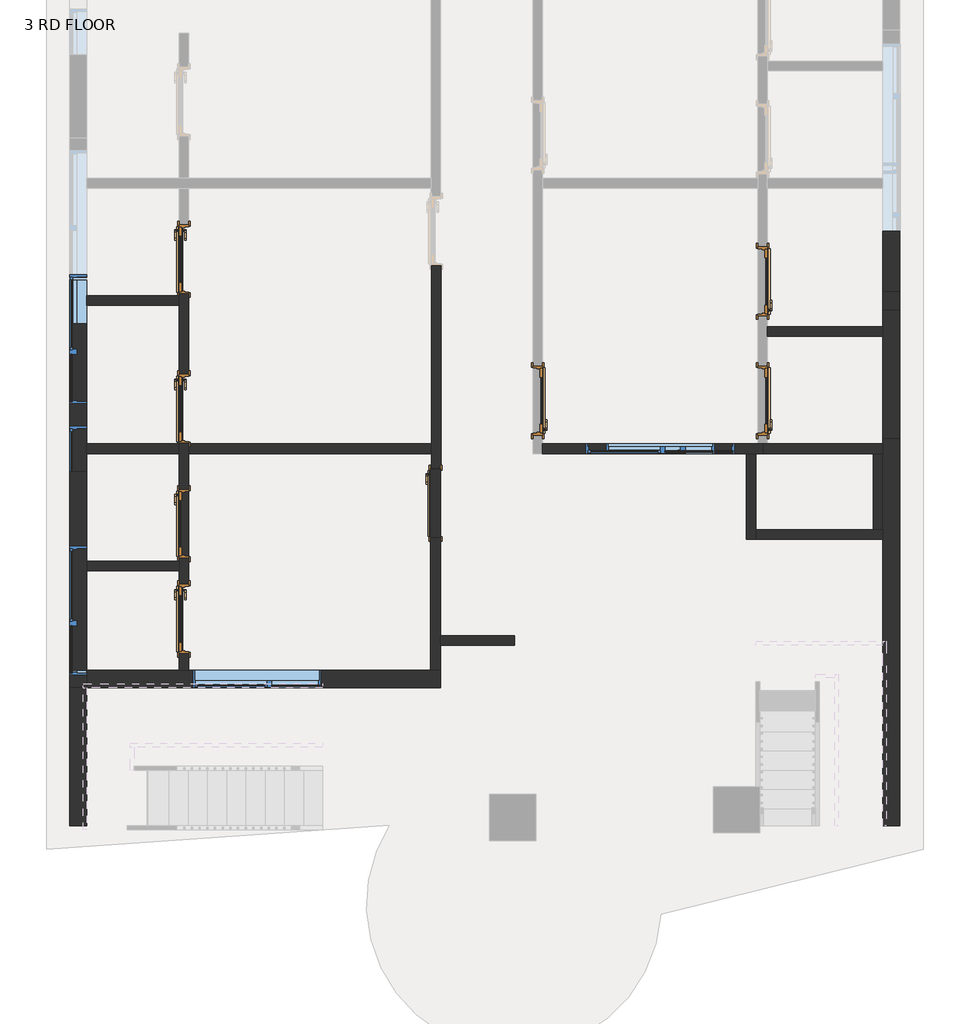
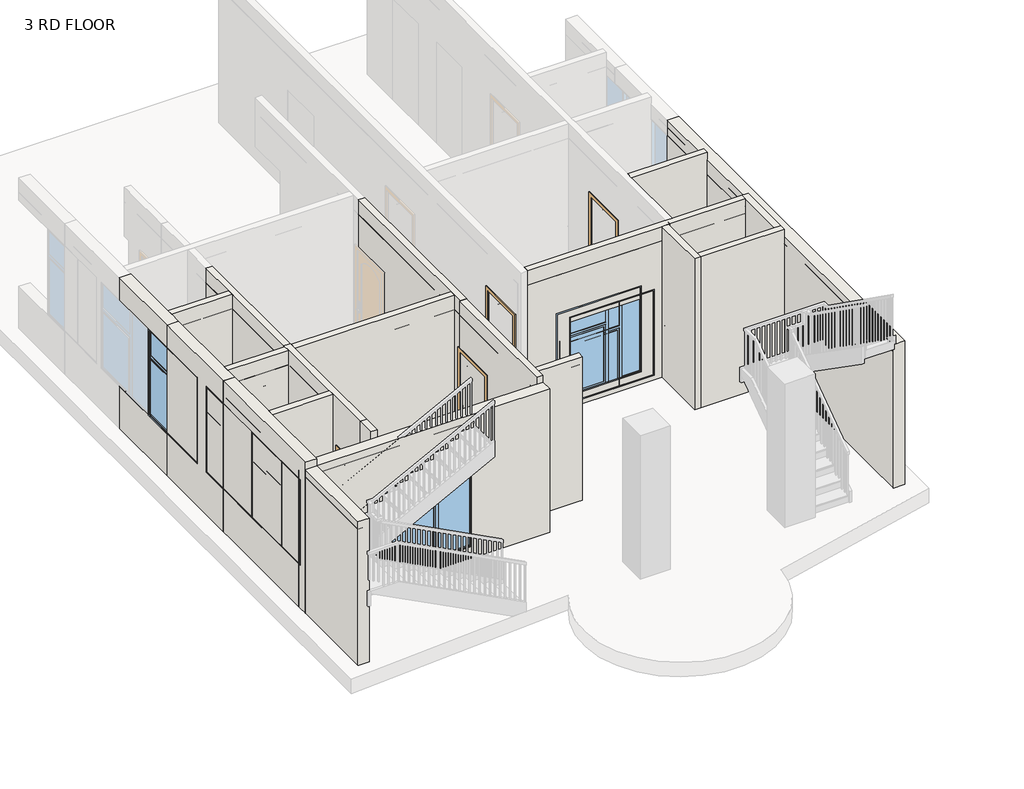
# One storey, part 1 of 5: 41 walls, 8 doors, 7 windows.
"""IFC4 building model written with IfcOpenShell, lengths in millimetres."""

from ifc_helpers import new_model, si_unit, frame, origin, place, context, project, spatial, polyline, outline, extrude, faceted_brep, transform, mapped, element, save
from components import door_346b4a94, m_window_casement_double_sidelight_1702_x_1829mm_c8b42c7f, m_window_casement_double_sidelight_1702_x_1829mm_92594323

model = new_model("IFC4")

# Units and contexts
model_context = context("Model", 3, world=origin())
ifc_project = project(units=[si_unit("LENGTHUNIT", "METRE", prefix="MILLI")], contexts=[model_context])

# Site, building, storey
site = spatial("IfcSite", under=ifc_project)
building = spatial("IfcBuilding", under=site)
storey = spatial("IfcBuildingStorey", under=building, Name="3 RD FLOOR", Elevation=9601.2)

# Doors
placement = place(None, origin())
door_shape = door_346b4a94(model_context)
element("IfcDoor", 1, ObjectType="2'10\"X7'", at=placement, inside=storey, context=model_context, shape_type="MappedRepresentation", body=[
    mapped(door_shape, transform((2698.7641134, -459.3600272, 9601.2), x_axis=(0.0, -1.0, 0.0), y_axis=(1.0, 0.0, 0.0), z_axis=(0.0, 0.0, 1.0))),
])
element("IfcDoor", 2, ObjectType="2'10\"X7'", at=placement, inside=storey, context=model_context, shape_type="MappedRepresentation", body=[
    mapped(door_shape, transform((2698.7641134, -2034.1600272, 9601.2), x_axis=(0.0, -1.0, 0.0), y_axis=(1.0, 0.0, 0.0), z_axis=(0.0, 0.0, 1.0))),
])
element("IfcDoor", 3, ObjectType="2'10\"X7'", at=placement, inside=storey, context=model_context, shape_type="MappedRepresentation", body=[
    mapped(door_shape, transform((-273.0358866, -2034.1600272, 9601.2), x_axis=(0.0, -1.0, 0.0), y_axis=(1.0, 0.0, 0.0), z_axis=(0.0, 0.0, 1.0))),
])
element("IfcDoor", 4, ObjectType="2'10\"X7'", at=placement, inside=storey, context=model_context, shape_type="MappedRepresentation", body=[
    mapped(door_shape, transform((-4952.9858866, -3659.7600272, 9601.2), x_axis=(0.0, 1.0, 0.0), y_axis=(-1.0, 0.0, 0.0), z_axis=(0.0, 0.0, 1.0))),
])
element("IfcDoor", 5, ObjectType="2'10\"X7'", at=placement, inside=storey, context=model_context, shape_type="MappedRepresentation", body=[
    mapped(door_shape, transform((-4952.9858866, -2142.5151651, 9601.2), x_axis=(0.0, 1.0, 0.0), y_axis=(-1.0, 0.0, 0.0), z_axis=(0.0, 0.0, 1.0))),
])
element("IfcDoor", 6, ObjectType="2'10\"X7'", at=placement, inside=storey, context=model_context, shape_type="MappedRepresentation", body=[
    mapped(door_shape, transform((-4952.9858866, -167.9704957, 9601.2), x_axis=(0.0, 1.0, 0.0), y_axis=(-1.0, 0.0, 0.0), z_axis=(0.0, 0.0, 1.0))),
])
element("IfcDoor", 7, ObjectType="2'10\"X7'", at=placement, inside=storey, context=model_context, shape_type="MappedRepresentation", body=[
    mapped(door_shape, transform((-1629.1419858, -3390.4626067, 9601.2), x_axis=(0.0, 1.0, 0.0), y_axis=(-1.0, 0.0, 0.0), z_axis=(0.0, 0.0, 1.0))),
])
element("IfcDoor", 8, ObjectType="2'10\"X7'", at=placement, inside=storey, context=model_context, shape_type="MappedRepresentation", body=[
    mapped(door_shape, transform((-4952.9858866, -4917.0600272, 9601.2), x_axis=(0.0, 1.0, 0.0), y_axis=(-1.0, 0.0, 0.0), z_axis=(0.0, 0.0, 1.0))),
])

# Walls
element("IfcWall", 9, ObjectType="Generic - 4.5\"", at=placement, inside=storey, context=model_context, shape_type="SweptSolid", body=[
    extrude(outline(polyline([(-5013.3108866, -776.8600272), (-6232.5508078, -776.8600272), (-6232.5508078, -649.8600272), (-5013.3108866, -649.8600272), (-5013.3108866, -776.8600272)])), frame((0.0, 0.0, 9601.2), z_axis=(0.0, 0.0, 1.0), x_axis=(1.0, 0.0, 0.0)), (0.0, 0.0, 1.0), 3200.4),
])
element("IfcWall", 10, ObjectType="Generic - 4.5\"", at=placement, inside=storey, context=model_context, shape_type="Brep", body=[
    faceted_brep([(-5013.3108866, -2574.3151651, 12801.6), (-5013.3108866, -776.8600272, 12801.6), (-5013.3108866, -649.8600272, 12801.6), (-5013.3108866, 136.8295043, 12801.6), (-5013.3108866, 136.8295043, 12496.8), (-5013.3108866, 136.8295043, 11759.8), (-5013.3108866, -624.7704957, 11759.8), (-5013.3108866, -624.7704957, 9601.2), (-5013.3108866, -649.8600272, 9601.2), (-5013.3108866, -776.8600272, 9601.2), (-5013.3108866, -1685.7151651, 9601.2), (-5013.3108866, -1685.7151651, 11759.8), (-5013.3108866, -2574.3151651, 11759.8), (-5013.3108866, -2574.3151651, 12496.8), (-4886.3108866, 136.8295043, 12801.6), (-4886.3108866, -2574.3151651, 12801.6), (-4886.3108866, -2574.3151651, 12496.8), (-4886.3108866, -2574.3151651, 11759.8), (-4886.3108866, -1685.7151651, 11759.8), (-4886.3108866, -1685.7151651, 9601.2), (-4886.3108866, -624.7704957, 9601.2), (-4886.3108866, -624.7704957, 11759.8), (-4886.3108866, 136.8295043, 11759.8), (-4886.3108866, 136.8295043, 12496.8)], [[[0, 1, 2, 3, 4, 5, 6, 7, 8, 9, 10, 11, 12, 13]], [[14, 15, 16, 17, 18, 19, 20, 21, 22, 23]], [[19, 10, 9, 8, 7, 20]], [[3, 2, 1, 0, 15, 14]], [[18, 11, 10, 19]], [[11, 18, 17, 12]], [[21, 6, 5, 22]], [[6, 21, 20, 7]], [[15, 0, 13, 12, 17, 16]], [[3, 14, 23, 22, 5, 4]]]),
])
element("IfcWall", 11, ObjectType="Generic - 4.5\"", at=placement, inside=storey, context=model_context, shape_type="SweptSolid", body=[
    extrude(outline(polyline([(-5013.3108866, -2732.6600272), (-6232.5508078, -2732.6600272), (-6232.5508078, -2605.6600272), (-5013.3108866, -2605.6600272), (-5013.3108866, -2732.6600272)])), frame((0.0, 0.0, 9601.2), z_axis=(0.0, 0.0, 1.0), x_axis=(1.0, 0.0, 0.0)), (0.0, 0.0, 1.0), 3200.4),
])
element("IfcWall", 12, ObjectType="Generic - 4.5\"", at=placement, inside=storey, context=model_context, shape_type="Brep", body=[
    faceted_brep([(-5013.3108866, -5221.8600272, 12801.6), (-5013.3108866, -4282.0600272, 12801.6), (-5013.3108866, -4155.0600272, 12801.6), (-5013.3108866, -2732.6600272, 12801.6), (-5013.3108866, -2605.6600272, 12801.6), (-5013.3108866, -2574.3151651, 12801.6), (-5013.3108866, -2574.3151651, 12496.8), (-5013.3108866, -2574.3151651, 11759.8), (-5013.3108866, -2599.3151651, 11759.8), (-5013.3108866, -2599.3151651, 9601.2), (-5013.3108866, -2605.6600272, 9601.2), (-5013.3108866, -2732.6600272, 9601.2), (-5013.3108866, -3202.9600272, 9601.2), (-5013.3108866, -3202.9600272, 11759.8), (-5013.3108866, -4116.5600272, 11759.8), (-5013.3108866, -4116.5600272, 9601.2), (-5013.3108866, -4155.0600272, 9601.2), (-5013.3108866, -4282.0600272, 9601.2), (-5013.3108866, -4460.2600272, 9601.2), (-5013.3108866, -4460.2600272, 11759.8), (-5013.3108866, -5221.8600272, 11759.8), (-5013.3108866, -5221.8600272, 12496.8), (-4886.3108866, -2574.3151651, 12801.6), (-4886.3108866, -2605.6600272, 12801.6), (-4886.3108866, -2732.6600272, 12801.6), (-4886.3108866, -5221.8600272, 12801.6), (-4886.3108866, -5221.8600272, 12496.8), (-4886.3108866, -5221.8600272, 11759.8), (-4886.3108866, -4460.2600272, 11759.8), (-4886.3108866, -4460.2600272, 9601.2), (-4886.3108866, -4116.5600272, 9601.2), (-4886.3108866, -4116.5600272, 11759.8), (-4886.3108866, -3202.9600272, 11759.8), (-4886.3108866, -3202.9600272, 9601.2), (-4886.3108866, -2732.6600272, 9601.2), (-4886.3108866, -2605.6600272, 9601.2), (-4886.3108866, -2599.3151651, 9601.2), (-4886.3108866, -2599.3151651, 11759.8), (-4886.3108866, -2574.3151651, 11759.8), (-4886.3108866, -2574.3151651, 12496.8)], [[[0, 1, 2, 3, 4, 5, 6, 7, 8, 9, 10, 11, 12, 13, 14, 15, 16, 17, 18, 19, 20, 21]], [[22, 23, 24, 25, 26, 27, 28, 29, 30, 31, 32, 33, 34, 35, 36, 37, 38, 39]], [[33, 12, 11, 10, 9, 36, 35, 34]], [[15, 30, 29, 18, 17, 16]], [[5, 4, 3, 2, 1, 0, 25, 24, 23, 22]], [[32, 13, 12, 33]], [[13, 32, 31, 14]], [[14, 31, 30, 15]], [[37, 8, 7, 38]], [[8, 37, 36, 9]], [[28, 19, 18, 29]], [[19, 28, 27, 20]], [[5, 22, 39, 38, 7, 6]], [[25, 0, 21, 20, 27, 26]]]),
])
element("IfcWall", 13, ObjectType="Generic - 4.5\"", at=placement, inside=storey, context=model_context, shape_type="SweptSolid", body=[
    extrude(outline(polyline([(-5013.3108866, -4282.0600272), (-6232.5324766, -4282.0600272), (-6232.5342541, -4155.0600272), (-5013.3108866, -4155.0600272), (-5013.3108866, -4282.0600272)])), frame((0.0, 0.0, 9601.2), z_axis=(0.0, 0.0, 1.0), x_axis=(1.0, 0.0, 0.0)), (0.0, 0.0, 1.0), 3200.4),
])
element("IfcWall", 14, ObjectType="Generic - 4.5\"", at=placement, inside=storey, context=model_context, shape_type="SweptSolid", body=[
    extrude(outline(polyline([(-1685.9108866, -2732.6600272), (-4886.3108866, -2732.6600272), (-4886.3108866, -2605.6600272), (-1685.9108866, -2605.6600272), (-1685.9108866, -2732.6600272)])), frame((0.0, 0.0, 9601.2), z_axis=(0.0, 0.0, 1.0), x_axis=(1.0, 0.0, 0.0)), (0.0, 0.0, 1.0), 3200.4),
])
element("IfcWall", 15, ObjectType="Generic - 4.5\"", at=placement, inside=storey, context=model_context, shape_type="Brep", body=[
    faceted_brep([(-1680.4827262, -2933.2626067, 12801.6), (-1680.4827262, 609.3637706, 12801.6), (-1680.4827262, 609.3637706, 11759.8), (-1680.4827262, -253.8362294, 11759.8), (-1680.4827262, -253.8362294, 9601.2), (-1680.4827262, -2933.2626067, 9601.2), (-1553.4827262, 609.3637706, 12801.6), (-1553.4827262, -2933.2626067, 12801.6), (-1553.4827262, -2933.2626067, 9601.2), (-1553.4827262, -253.8362294, 9601.2), (-1553.4827262, -253.8362294, 11759.8), (-1553.4827262, 609.3637706, 11759.8), (-1562.4669858, -2933.2626067, 9601.2), (-1562.4669858, -2933.2626067, 12801.6), (-1558.4871817, 609.3637706, 12801.6), (-1558.4871817, 609.3637706, 11759.8)], [[[0, 1, 2, 3, 4, 5]], [[6, 7, 8, 9, 10, 11]], [[8, 12, 5, 4, 9]], [[1, 0, 13, 7, 6, 14]], [[10, 3, 2, 15, 11]], [[3, 10, 9, 4]], [[5, 12, 8, 7, 13, 0]], [[1, 14, 6, 11, 15, 2]]]),
])
element("IfcWall", 16, ObjectType="Generic - 4.5\"", at=placement, inside=storey, context=model_context, shape_type="Brep", body=[
    faceted_brep([(-1689.4669858, -5596.1082131, 12801.6), (-1689.4669858, -2933.2626067, 12801.6), (-1689.4669858, -2933.2626067, 9601.2), (-1689.4669858, -2933.6626067, 9601.2), (-1689.4669858, -2933.6626067, 11759.8), (-1689.4669858, -3847.2626067, 11759.8), (-1689.4669858, -3847.2626067, 9601.2), (-1689.4669858, -5596.1082131, 9601.2), (-1562.4669858, -2933.2626067, 12801.6), (-1562.4669858, -5596.1082131, 12801.6), (-1562.4669858, -5596.1082131, 12649.2), (-1562.4669858, -5596.1082131, 12496.8), (-1562.4669858, -5596.1082131, 9601.2), (-1562.4669858, -5263.3822004, 9601.2), (-1562.4669858, -5136.3822004, 9601.2), (-1562.4669858, -3847.2626067, 9601.2), (-1562.4669858, -3847.2626067, 11759.8), (-1562.4669858, -2933.6626067, 11759.8), (-1562.4669858, -2933.6626067, 9601.2), (-1562.4669858, -2933.2626067, 9601.2), (-1680.4827262, -2933.2626067, 9601.2), (-1680.4827262, -2933.2626067, 12801.6)], [[[0, 1, 2, 3, 4, 5, 6, 7]], [[8, 9, 10, 11, 12, 13, 14, 15, 16, 17, 18, 19]], [[2, 20, 19, 18, 3]], [[12, 7, 6, 15, 14, 13]], [[1, 0, 9, 8, 21]], [[17, 4, 3, 18]], [[4, 17, 16, 5]], [[5, 16, 15, 6]], [[7, 12, 11, 10, 9, 0]], [[1, 21, 8, 19, 20, 2]]]),
])
element("IfcWall", 17, ObjectType="Generic - 4.5\"", at=placement, inside=storey, context=model_context, shape_type="Brep", body=[
    faceted_brep([(-212.7108866, -2732.6600272, 12801.6), (-212.7108866, -2732.6600272, 9601.2), (2479.6891134, -2732.6600272, 9601.2), (2606.6891134, -2732.6600272, 9601.2), (4281.7311655, -2732.6600272, 9601.2), (4281.7311655, -2732.6600272, 12649.2), (4154.7311655, -2732.6600272, 12649.2), (4154.7311655, -2732.6600272, 12801.6), (2606.6891134, -2732.6600272, 12801.6), (2479.6891134, -2732.6600272, 12801.6), (358.7891134, -2732.6600272, 11691.1092519), (2060.5891134, -2732.6600272, 11691.1092519), (2060.5891134, -2732.6600272, 9862.3092519), (358.7891134, -2732.6600272, 9862.3092519), (-212.7108866, -2605.6600272, 9601.2), (-212.7108866, -2605.6600272, 12801.6), (2632.0891134, -2605.6600272, 12801.6), (2759.0891134, -2605.6600272, 12801.6), (4154.7311655, -2605.6600272, 12801.6), (4154.7311655, -2605.6600272, 12649.2), (4281.7311655, -2605.6600272, 12649.2), (4281.7311655, -2605.6600272, 9601.2), (2759.0891134, -2605.6600272, 9601.2), (2632.0891134, -2605.6600272, 9601.2), (358.7891134, -2605.6600272, 11691.1092519), (358.7891134, -2605.6600272, 9862.3092519), (2060.5891134, -2605.6600272, 9862.3092519), (2060.5891134, -2605.6600272, 11691.1092519)], [[[0, 1, 2, 3, 4, 5, 6, 7, 8, 9], [10, 11, 12, 13]], [[14, 15, 16, 17, 18, 19, 20, 21, 22, 23], [24, 25, 26, 27]], [[4, 3, 2, 1, 14, 23, 22, 21]], [[0, 9, 8, 7, 18, 17, 16, 15]], [[25, 24, 10, 13]], [[26, 25, 13, 12]], [[27, 26, 12, 11]], [[24, 27, 11, 10]], [[0, 15, 14, 1]], [[19, 6, 5, 20]], [[4, 21, 20, 5]], [[7, 6, 19, 18]]]),
])
element("IfcWall", 18, ObjectType="Generic - 4.5\"", at=placement, inside=storey, context=model_context, shape_type="SweptSolid", body=[
    extrude(outline(polyline([(4281.7311655, -1183.2600272), (2759.0891134, -1183.2600272), (2759.0891134, -1056.2600272), (4281.7311655, -1056.2600272), (4281.7311655, -1183.2600272)])), frame((0.0, 0.0, 9601.2), z_axis=(0.0, 0.0, 1.0), x_axis=(1.0, 0.0, 0.0)), (0.0, 0.0, 1.0), 3200.4),
])
element("IfcWall", 19, ObjectType="Generic - 4.5\"", at=placement, inside=storey, context=model_context, shape_type="SweptSolid", body=[
    extrude(outline(polyline([(-5013.3108866, -776.8600272), (-6232.5508078, -776.8600272), (-6232.5508078, -649.8600272), (-5013.3108866, -649.8600272), (-5013.3108866, -776.8600272)])), frame((0.0, 0.0, 9601.2), z_axis=(0.0, 0.0, 1.0), x_axis=(1.0, 0.0, 0.0)), (0.0, 0.0, 1.0), 2895.6),
])
element("IfcWall", 20, ObjectType="Generic - 4.5\"", at=placement, inside=storey, context=model_context, shape_type="Brep", body=[
    faceted_brep([(-5013.3108866, -2574.3151651, 12496.8), (-5013.3108866, -776.8600272, 12496.8), (-5013.3108866, -649.8600272, 12496.8), (-5013.3108866, 136.8295043, 12496.8), (-5013.3108866, 136.8295043, 11759.8), (-5013.3108866, -624.7704957, 11759.8), (-5013.3108866, -624.7704957, 9601.2), (-5013.3108866, -649.8600272, 9601.2), (-5013.3108866, -776.8600272, 9601.2), (-5013.3108866, -1685.7151651, 9601.2), (-5013.3108866, -1685.7151651, 11759.8), (-5013.3108866, -2574.3151651, 11759.8), (-4886.3108866, 136.8295043, 12496.8), (-4886.3108866, -2574.3151651, 12496.8), (-4886.3108866, -2574.3151651, 11759.8), (-4886.3108866, -1685.7151651, 11759.8), (-4886.3108866, -1685.7151651, 9601.2), (-4886.3108866, -624.7704957, 9601.2), (-4886.3108866, -624.7704957, 11759.8), (-4886.3108866, 136.8295043, 11759.8)], [[[0, 1, 2, 3, 4, 5, 6, 7, 8, 9, 10, 11]], [[12, 13, 14, 15, 16, 17, 18, 19]], [[16, 9, 8, 7, 6, 17]], [[13, 0, 11, 14]], [[3, 12, 19, 4]], [[3, 2, 1, 0, 13, 12]], [[18, 5, 4, 19]], [[5, 18, 17, 6]], [[15, 10, 9, 16]], [[10, 15, 14, 11]]]),
])
element("IfcWall", 21, ObjectType="Generic - 4.5\"", at=placement, inside=storey, context=model_context, shape_type="SweptSolid", body=[
    extrude(outline(polyline([(-5013.3108866, -2732.6600272), (-6232.5508078, -2732.6600272), (-6232.5508078, -2605.6600272), (-5013.3108866, -2605.6600272), (-5013.3108866, -2732.6600272)])), frame((0.0, 0.0, 9601.2), z_axis=(0.0, 0.0, 1.0), x_axis=(1.0, 0.0, 0.0)), (0.0, 0.0, 1.0), 2895.6),
])
element("IfcWall", 22, ObjectType="Generic - 4.5\"", at=placement, inside=storey, context=model_context, shape_type="Brep", body=[
    faceted_brep([(-5013.3108866, -5221.8600272, 12496.8), (-5013.3108866, -4282.0600272, 12496.8), (-5013.3108866, -4155.0600272, 12496.8), (-5013.3108866, -2732.6600272, 12496.8), (-5013.3108866, -2605.6600272, 12496.8), (-5013.3108866, -2574.3151651, 12496.8), (-5013.3108866, -2574.3151651, 11759.8), (-5013.3108866, -2599.3151651, 11759.8), (-5013.3108866, -2599.3151651, 9601.2), (-5013.3108866, -2605.6600272, 9601.2), (-5013.3108866, -2732.6600272, 9601.2), (-5013.3108866, -4155.0600272, 9601.2), (-5013.3108866, -4282.0600272, 9601.2), (-5013.3108866, -4460.2600272, 9601.2), (-5013.3108866, -4460.2600272, 11759.8), (-5013.3108866, -5221.8600272, 11759.8), (-4886.3108866, -2574.3151651, 12496.8), (-4886.3108866, -2605.6600272, 12496.8), (-4886.3108866, -2732.6600272, 12496.8), (-4886.3108866, -5221.8600272, 12496.8), (-4886.3108866, -5221.8600272, 11759.8), (-4886.3108866, -4460.2600272, 11759.8), (-4886.3108866, -4460.2600272, 9601.2), (-4886.3108866, -2732.6600272, 9601.2), (-4886.3108866, -2605.6600272, 9601.2), (-4886.3108866, -2599.3151651, 9601.2), (-4886.3108866, -2599.3151651, 11759.8), (-4886.3108866, -2574.3151651, 11759.8)], [[[0, 1, 2, 3, 4, 5, 6, 7, 8, 9, 10, 11, 12, 13, 14, 15]], [[16, 17, 18, 19, 20, 21, 22, 23, 24, 25, 26, 27]], [[8, 25, 24, 23, 22, 13, 12, 11, 10, 9]], [[19, 0, 15, 20]], [[5, 16, 27, 6]], [[5, 4, 3, 2, 1, 0, 19, 18, 17, 16]], [[21, 14, 13, 22]], [[14, 21, 20, 15]], [[26, 7, 6, 27]], [[7, 26, 25, 8]]]),
])
element("IfcWall", 23, ObjectType="Generic - 4.5\"", at=placement, inside=storey, context=model_context, shape_type="SweptSolid", body=[
    extrude(outline(polyline([(-5013.3108866, -4282.0600272), (-6232.5324766, -4282.0600272), (-6232.5342541, -4155.0600272), (-5013.3108866, -4155.0600272), (-5013.3108866, -4282.0600272)])), frame((0.0, 0.0, 9601.2), z_axis=(0.0, 0.0, 1.0), x_axis=(1.0, 0.0, 0.0)), (0.0, 0.0, 1.0), 2895.6),
])
element("IfcWall", 24, ObjectType="Generic - 4.5\"", at=placement, inside=storey, context=model_context, shape_type="SweptSolid", body=[
    extrude(outline(polyline([(-1685.9108866, -2732.6600272), (-4886.3108866, -2732.6600272), (-4886.3108866, -2605.6600272), (-1685.9108866, -2605.6600272), (-1685.9108866, -2732.6600272)])), frame((0.0, 0.0, 9601.2), z_axis=(0.0, 0.0, 1.0), x_axis=(1.0, 0.0, 0.0)), (0.0, 0.0, 1.0), 2895.6),
])
element("IfcWall", 25, ObjectType="Generic - 4.5\"", at=placement, inside=storey, context=model_context, shape_type="Brep", body=[
    faceted_brep([(-1680.4827262, -2933.2626067, 9601.2), (-1680.4827262, -2933.2626067, 12496.8), (-1680.4827262, 609.3637706, 12496.8), (-1680.4827262, 609.3637706, 11759.8), (-1680.4827262, -253.8362294, 11759.8), (-1680.4827262, -253.8362294, 9601.2), (-1553.4827262, -2933.2626067, 12496.8), (-1553.4827262, -2933.2626067, 9601.2), (-1553.4827262, -253.8362294, 9601.2), (-1553.4827262, -253.8362294, 11759.8), (-1553.4827262, 609.3637706, 11759.8), (-1553.4827262, 609.3637706, 12496.8), (-1562.4669858, -2933.2626067, 9601.2), (-1562.4669858, -2933.2626067, 12496.8), (-1558.4871817, 609.3637706, 12496.8), (-1558.4871817, 609.3637706, 11759.8)], [[[0, 1, 2, 3, 4, 5]], [[6, 7, 8, 9, 10, 11]], [[7, 12, 0, 5, 8]], [[1, 0, 12, 7, 6, 13]], [[2, 14, 11, 10, 15, 3]], [[2, 1, 13, 6, 11, 14]], [[9, 4, 3, 15, 10]], [[4, 9, 8, 5]]]),
])
element("IfcWall", 26, ObjectType="Generic - 4.5\"", at=placement, inside=storey, context=model_context, shape_type="Brep", body=[
    faceted_brep([(-1689.4669858, -2933.2626067, 9601.2), (-1689.4669858, -5596.1082131, 9601.2), (-1689.4669858, -5596.1082131, 12496.8), (-1689.4669858, -2933.2626067, 12496.8), (-1562.4669858, -2933.2626067, 9601.2), (-1562.4669858, -2933.2626067, 12496.8), (-1562.4669858, -5136.3822004, 12496.8), (-1562.4669858, -5263.3822004, 12496.8), (-1562.4669858, -5596.1082131, 12496.8), (-1562.4669858, -5596.1082131, 9601.2), (-1562.4669858, -5263.3822004, 9601.2), (-1562.4669858, -5136.3822004, 9601.2), (-1680.4827262, -2933.2626067, 9601.2), (-1680.4827262, -2933.2626067, 12496.8)], [[[0, 1, 2, 3]], [[4, 5, 6, 7, 8, 9, 10, 11]], [[1, 0, 12, 4, 11, 10, 9]], [[0, 3, 13, 5, 4, 12]], [[3, 2, 8, 7, 6, 5, 13]], [[2, 1, 9, 8]]]),
])
element("IfcWall", 27, ObjectType="Generic - 4.5\"", at=placement, inside=storey, context=model_context, shape_type="Brep", body=[
    faceted_brep([(4281.7311655, -2732.6600272, 9601.2), (4281.7311655, -2732.6600272, 12496.8), (-212.7108866, -2732.6600272, 12496.8), (-212.7108866, -2732.6600272, 9601.2), (625.4891134, -2732.6600272, 9601.2), (625.4891134, -2732.6600272, 11415.3114654), (2327.2891134, -2732.6600272, 11415.3114654), (2327.2891134, -2732.6600272, 9601.2), (2479.6891134, -2732.6600272, 9601.2), (2606.6891134, -2732.6600272, 9601.2), (4281.7311655, -2605.6600272, 12496.8), (4281.7311655, -2605.6600272, 9601.2), (2759.0891134, -2605.6600272, 9601.2), (2632.0891134, -2605.6600272, 9601.2), (2327.2891134, -2605.6600272, 9601.2), (2327.2891134, -2605.6600272, 11415.3114654), (625.4891134, -2605.6600272, 11415.3114654), (625.4891134, -2605.6600272, 9601.2), (-212.7108866, -2605.6600272, 9601.2), (-212.7108866, -2605.6600272, 12496.8), (2632.0891134, -2605.6600272, 12496.8), (2759.0891134, -2605.6600272, 12496.8)], [[[0, 1, 2, 3, 4, 5, 6, 7, 8, 9]], [[10, 11, 12, 13, 14, 15, 16, 17, 18, 19, 20, 21]], [[3, 18, 17, 4]], [[11, 0, 9, 8, 7, 14, 13, 12]], [[1, 0, 11, 10]], [[2, 1, 10, 21, 20, 19]], [[16, 5, 4, 17]], [[6, 15, 14, 7]], [[5, 16, 15, 6]], [[3, 2, 19, 18]]]),
])
element("IfcWall", 28, ObjectType="Generic - 4.5\"", at=placement, inside=storey, context=model_context, shape_type="SweptSolid", body=[
    extrude(outline(polyline([(4281.7311655, -1183.2600272), (2759.0891134, -1183.2600272), (2759.0891134, -1056.2600272), (4281.7311655, -1056.2600272), (4281.7311655, -1183.2600272)])), frame((0.0, 0.0, 9601.2), z_axis=(0.0, 0.0, 1.0), x_axis=(1.0, 0.0, 0.0)), (0.0, 0.0, 1.0), 2895.6),
])
element("IfcWall", 29, ObjectType="Generic - 4.5\"", at=placement, inside=storey, context=model_context, shape_type="Brep", body=[
    faceted_brep([(-212.7108866, -2732.6600272, 9601.2), (2479.6891134, -2732.6600272, 9601.2), (2606.6891134, -2732.6600272, 9601.2), (2695.5891134, -2732.6600272, 9601.2), (2695.5891134, -2732.6600272, 12496.8), (2632.0891134, -2732.6600272, 12496.8), (-212.7108866, -2732.6600272, 12496.8), (625.4891134, -2732.6600272, 11527.1883506), (2327.2891134, -2732.6600272, 11527.1883506), (2327.2891134, -2732.6600272, 9698.3883506), (625.4891134, -2732.6600272, 9698.3883506), (-212.7108866, -2605.6600272, 9601.2), (-212.7108866, -2605.6600272, 12496.8), (2632.0891134, -2605.6600272, 12496.8), (2695.5891134, -2605.6600272, 12496.8), (2695.5891134, -2605.6600272, 9601.2), (2632.0891134, -2605.6600272, 9601.2), (625.4891134, -2605.6600272, 11527.1883506), (625.4891134, -2605.6600272, 9698.3883506), (2327.2891134, -2605.6600272, 9698.3883506), (2327.2891134, -2605.6600272, 11527.1883506)], [[[0, 1, 2, 3, 4, 5, 6], [7, 8, 9, 10]], [[11, 12, 13, 14, 15, 16], [17, 18, 19, 20]], [[3, 2, 1, 0, 11, 16, 15]], [[4, 3, 15, 14]], [[6, 5, 4, 14, 13, 12]], [[18, 17, 7, 10]], [[19, 18, 10, 9]], [[20, 19, 9, 8]], [[17, 20, 8, 7]], [[0, 6, 12, 11]]]),
])
element("IfcWall", 30, ObjectType="Generic - 5\"", at=placement, inside=storey, context=model_context, shape_type="Brep", body=[
    faceted_brep([(-5013.3108866, -5593.5822004, 9601.2), (-5013.3108866, -5593.5822004, 12801.6), (-5013.3108866, -5221.8600272, 12801.6), (-5013.3108866, -5221.8600272, 12496.8), (-5013.3108866, -5221.8600272, 11759.8), (-5013.3108866, -5373.8600272, 11759.8), (-5013.3108866, -5373.8600272, 9601.2), (-4886.3108866, -5593.5822004, 12801.6), (-4886.3108866, -5593.5822004, 9601.2), (-4886.3108866, -5373.8600272, 9601.2), (-4886.3108866, -5373.8600272, 11759.8), (-4886.3108866, -5221.8600272, 11759.8), (-4886.3108866, -5221.8600272, 12496.8), (-4886.3108866, -5221.8600272, 12801.6)], [[[0, 1, 2, 3, 4, 5, 6]], [[7, 8, 9, 10, 11, 12, 13]], [[8, 0, 6, 9]], [[1, 0, 8, 7]], [[2, 1, 7, 13]], [[10, 5, 4, 11]], [[5, 10, 9, 6]], [[2, 13, 12, 11, 4, 3]]]),
])
element("IfcWall", 31, ObjectType="Generic - 5\"", at=placement, inside=storey, context=model_context, shape_type="SweptSolid", body=[
    extrude(outline(polyline([(-1562.4669858, -5136.3822004), (-581.0108866, -5136.3822004), (-581.0108866, -5263.3822004), (-1562.4669858, -5263.3822004), (-1562.4669858, -5136.3822004)])), frame((0.0, 0.0, 9601.2), z_axis=(0.0, 0.0, 1.0), x_axis=(1.0, 0.0, 0.0)), (0.0, 0.0, 1.0), 3048.0),
])
element("IfcWall", 32, ObjectType="Generic - 5\"", at=placement, inside=storey, context=model_context, shape_type="SweptSolid", body=[
    extrude(outline(polyline([(-5593.5822004, 9601.2), (-5593.5822004, 12496.8), (-5221.8600272, 12496.8), (-5221.8600272, 11759.8), (-5373.8600272, 11759.8), (-5373.8600272, 9601.2), (-5593.5822004, 9601.2)])), frame((-5013.3108866, 0.0, 0.0), z_axis=(1.0, 0.0, 0.0), x_axis=(0.0, 1.0, 0.0)), (0.0, 0.0, 1.0), 127.0),
])
element("IfcWall", 33, ObjectType="Generic - 5\"", at=placement, inside=storey, context=model_context, shape_type="SweptSolid", body=[
    extrude(outline(polyline([(-1562.4669858, -5136.3822004), (-581.0108866, -5136.3822004), (-581.0108866, -5263.3822004), (-1562.4669858, -5263.3822004), (-1562.4669858, -5136.3822004)])), frame((0.0, 0.0, 9601.2), z_axis=(0.0, 0.0, 1.0), x_axis=(1.0, 0.0, 0.0)), (0.0, 0.0, 1.0), 2895.6),
])
element("IfcWall", 34, ObjectType="Generic - 5\"", at=placement, inside=storey, context=model_context, shape_type="Brep", body=[
    faceted_brep([(2479.6891134, -2732.6600272, 12801.6), (2479.6891134, -2732.6600272, 9601.2), (2479.6891134, -3866.3822004, 9601.2), (2479.6891134, -3866.3822004, 12801.6), (2606.6891134, -2732.6600272, 9601.2), (2606.6891134, -2732.6600272, 12801.6), (2606.6891134, -3739.3822004, 12801.6), (2606.6891134, -3866.3822004, 12801.6), (2606.6891134, -3866.3822004, 9601.2), (2606.6891134, -3739.3822004, 9601.2)], [[[0, 1, 2, 3]], [[4, 5, 6, 7, 8, 9]], [[2, 1, 4, 9, 8]], [[0, 3, 7, 6, 5]], [[3, 2, 8, 7]], [[0, 5, 4, 1]]]),
])
element("IfcWall", 35, ObjectType="Generic - 5\"", at=placement, inside=storey, context=model_context, shape_type="Brep", body=[
    faceted_brep([(2606.6891134, -3866.3822004, 9601.2), (4281.7311655, -3866.3822004, 9601.2), (4281.7311655, -3866.3822004, 12801.6), (2606.6891134, -3866.3822004, 12801.6), (2606.6891134, -3739.3822004, 9601.2), (2606.6891134, -3739.3822004, 12801.6), (4154.7311655, -3739.3822004, 12801.6), (4281.7311655, -3739.3822004, 12801.6), (4281.7311655, -3739.3822004, 9601.2), (4154.7311655, -3739.3822004, 9601.2)], [[[0, 1, 2, 3]], [[4, 5, 6, 7, 8, 9]], [[1, 0, 4, 9, 8]], [[3, 2, 7, 6, 5]], [[0, 3, 5, 4]], [[2, 1, 8, 7]]]),
])
element("IfcWall", 36, ObjectType="Generic - 5\"", at=placement, inside=storey, context=model_context, shape_type="Brep", body=[
    faceted_brep([(4281.7311655, -3739.3822004, 9601.2), (4281.7311655, -2605.6600272, 9601.2), (4281.7311655, -2605.6600272, 12801.6), (4281.7311655, -3739.3822004, 12801.6), (4154.7311655, -3739.3822004, 9601.2), (4154.7311655, -3739.3822004, 12801.6), (4154.7311655, -2732.6600272, 12801.6), (4154.7311655, -2605.6600272, 12801.6), (4154.7311655, -2605.6600272, 12649.2), (4154.7311655, -2605.6600272, 9601.2), (4154.7311655, -2732.6600272, 9601.2)], [[[0, 1, 2, 3]], [[4, 5, 6, 7, 8, 9, 10]], [[1, 0, 4, 10, 9]], [[3, 2, 7, 6, 5]], [[0, 3, 5, 4]], [[1, 9, 8, 7, 2]]]),
])
element("IfcWall", 37, ObjectType="Generic - 5\"", at=placement, inside=storey, context=model_context, shape_type="Brep", body=[
    faceted_brep([(2695.5891134, -2732.6600272, 9601.2), (4154.7311655, -2732.6600272, 9601.2), (4154.7311655, -2732.6600272, 12801.6), (2632.0891134, -2732.6600272, 12801.6), (2632.0891134, -2732.6600272, 12496.8), (2695.5891134, -2732.6600272, 12496.8), (2695.5891134, -2605.6600272, 9601.2), (2695.5891134, -2605.6600272, 12496.8), (2632.0891134, -2605.6600272, 12496.8), (2632.0891134, -2605.6600272, 12801.6), (2759.0891134, -2605.6600272, 12801.6), (4154.7311655, -2605.6600272, 12801.6), (4154.7311655, -2605.6600272, 9601.2), (2759.0891134, -2605.6600272, 9601.2)], [[[0, 1, 2, 3, 4, 5]], [[6, 7, 8, 9, 10, 11, 12, 13]], [[1, 0, 6, 13, 12]], [[3, 2, 11, 10, 9]], [[2, 1, 12, 11]], [[0, 5, 7, 6]], [[4, 8, 7, 5]], [[4, 3, 9, 8]]]),
])
element("IfcWall", 38, ObjectType="Generic - 9\"", at=placement, inside=storey, context=model_context, shape_type="Brep", body=[
    faceted_brep([(4281.7311655, 200.5184135, 9601.2), (4281.7311655, -1056.2600272, 9601.2), (4281.7311655, -1183.2600272, 9601.2), (4281.7311655, -2605.6600272, 9601.2), (4281.7311655, -2732.6600272, 9601.2), (4281.7311655, -7650.9822004, 9601.2), (4281.7311655, -7650.9822004, 12649.2), (4281.7311655, -2732.6600272, 12649.2), (4281.7311655, -2605.6600272, 12649.2), (4281.7311655, 200.5184135, 12649.2), (4281.7311655, 200.5184135, 12330.0), (4281.7311655, -599.0600272, 12330.0), (4281.7311655, -599.0600272, 10501.2), (4281.7311655, 200.5184135, 10501.2), (4281.7311655, -2537.537179, 10501.2), (4281.7311655, -835.737179, 10501.2), (4281.7311655, -835.737179, 12330.0), (4281.7311655, -2537.537179, 12330.0), (4510.3311655, -7650.9822004, 9601.2), (4510.3311655, 200.5184135, 9601.2), (4510.3311655, 200.5184135, 10501.2), (4510.3311655, -599.0600272, 10501.2), (4510.3311655, -599.0600272, 12330.0), (4510.3311655, 200.5184135, 12330.0), (4510.3311655, 200.5184135, 12649.2), (4510.3311655, -7650.9822004, 12649.2), (4510.3311655, -835.737179, 10501.2), (4510.3311655, -2537.537179, 10501.2), (4510.3311655, -2537.537179, 12330.0), (4510.3311655, -835.737179, 12330.0), (4283.0918814, 200.5184135, 9601.2), (4283.0918814, 200.5184135, 12649.2), (4283.0918814, 200.5184135, 10501.2), (4283.0918814, 200.5184135, 12330.0)], [[[0, 1, 2, 3, 4, 5, 6, 7, 8, 9, 10, 11, 12, 13], [14, 15, 16, 17]], [[18, 19, 20, 21, 22, 23, 24, 25], [26, 27, 28, 29]], [[5, 4, 3, 2, 1, 0, 30, 19, 18]], [[6, 5, 18, 25]], [[9, 8, 7, 6, 25, 24, 31]], [[11, 22, 21, 12]], [[12, 21, 20, 32, 13]], [[22, 11, 10, 33, 23]], [[26, 15, 14, 27]], [[15, 26, 29, 16]], [[16, 29, 28, 17]], [[27, 14, 17, 28]], [[9, 31, 24, 23, 33, 10]], [[19, 30, 0, 13, 32, 20]]]),
])
element("IfcWall", 39, ObjectType="Generic - 9\"", at=placement, inside=storey, context=model_context, shape_type="Brep", body=[
    faceted_brep([(-6232.5108866, -5824.7082131, 9601.2), (-6232.5140859, -5596.1082131, 9601.2), (-6232.5324766, -4282.0600272, 9601.2), (-6232.5342541, -4155.0600272, 9601.2), (-6232.5508078, -2972.263382, 9601.2), (-6232.5508078, -2972.263382, 10501.2), (-6232.5131972, -5659.6082132, 10501.2), (-6232.5131972, -5659.6082132, 12330.0), (-6232.5508078, -2972.263382, 12330.0), (-6232.5508078, -2972.263382, 12496.8), (-6232.5508078, -2972.263382, 12801.6), (-6232.5342541, -4155.0600272, 12801.6), (-6232.5324766, -4282.0600272, 12801.6), (-6232.5108866, -5824.7082131, 12801.6), (-6232.5108866, -5824.7082131, 12649.2), (-6232.5108866, -5824.7082131, 12496.8), (-6461.1508078, -2972.2665814, 9601.2), (-6461.1108866, -5824.7082131, 9601.2), (-6461.1108866, -5824.7082131, 12496.8), (-6461.1108866, -5824.7082131, 12649.2), (-6461.1108866, -5824.7082131, 12801.6), (-6461.1508078, -2972.2665814, 12801.6), (-6461.1508078, -2972.2665814, 12496.8), (-6461.1508078, -2972.2665814, 12330.0), (-6461.1131972, -5659.6114126, 12330.0), (-6461.1131972, -5659.6114126, 10501.2), (-6461.1508078, -2972.2665814, 10501.2)], [[[0, 1, 2, 3, 4, 5, 6, 7, 8, 9, 10, 11, 12, 13, 14, 15]], [[16, 17, 18, 19, 20, 21, 22, 23, 24, 25, 26]], [[4, 3, 2, 1, 0, 17, 16]], [[13, 12, 11, 10, 21, 20]], [[5, 26, 25, 6]], [[23, 8, 7, 24]], [[24, 7, 6, 25]], [[13, 20, 19, 18, 17, 0, 15, 14]], [[4, 16, 26, 5]], [[21, 10, 9, 8, 23, 22]]]),
])
element("IfcWall", 40, ObjectType="Generic - 9\"", at=placement, inside=storey, context=model_context, shape_type="Brep", body=[
    faceted_brep([(-6232.5508078, -2972.2649817, 9601.2), (-6232.5508078, -2732.6600272, 9601.2), (-6232.5508078, -2605.6600272, 9601.2), (-6232.5508078, -1019.7048138, 9601.2), (-6232.5508078, -1019.7048138, 10501.2), (-6232.5508078, -2073.8048138, 10501.2), (-6232.5508078, -2073.8048138, 12330.0), (-6232.5508078, -1019.7048138, 12330.0), (-6232.5508078, -1019.7048138, 12496.8), (-6232.5508078, -1019.7048138, 12801.6), (-6232.5508078, -2605.6600272, 12801.6), (-6232.5508078, -2732.6600272, 12801.6), (-6232.5508078, -2972.2649817, 12801.6), (-6232.5508078, -2972.2649817, 12330.0), (-6232.5508078, -2375.3633819, 12330.0), (-6232.5508078, -2375.3633819, 10501.2), (-6232.5508078, -2972.2649817, 10501.2), (-6461.1508078, -1019.7048138, 9601.2), (-6461.1508078, -2972.2649817, 9601.2), (-6461.1508078, -2972.2649817, 10501.2), (-6461.1508078, -2375.3665813, 10501.2), (-6461.1508078, -2375.3665813, 12330.0), (-6461.1508078, -2972.2649817, 12330.0), (-6461.1508078, -2972.2649817, 12801.6), (-6461.1508078, -1019.7048138, 12801.6), (-6461.1508078, -1019.7048138, 12496.8), (-6461.1508078, -1019.7048138, 12330.0), (-6461.1508078, -2073.8048138, 12330.0), (-6461.1508078, -2073.8048138, 10501.2), (-6461.1508078, -1019.7048138, 10501.2)], [[[0, 1, 2, 3, 4, 5, 6, 7, 8, 9, 10, 11, 12, 13, 14, 15, 16]], [[17, 18, 19, 20, 21, 22, 23, 24, 25, 26, 27, 28, 29]], [[3, 2, 1, 0, 18, 17]], [[12, 11, 10, 9, 24, 23]], [[28, 5, 4, 29]], [[5, 28, 27, 6]], [[6, 27, 26, 7]], [[14, 21, 20, 15]], [[15, 20, 19, 16]], [[21, 14, 13, 22]], [[12, 23, 22, 13]], [[18, 0, 16, 19]], [[24, 9, 8, 7, 26, 25]], [[3, 17, 29, 4]]]),
])
element("IfcWall", 41, ObjectType="Generic - 9\"", at=placement, inside=storey, context=model_context, shape_type="Brep", body=[
    faceted_brep([(-6232.5508078, -1019.7048138, 9601.2), (-6232.5508078, -776.8600272, 9601.2), (-6232.5508078, -649.8600272, 9601.2), (-6232.5508078, 642.0011338, 9601.2), (-6232.5508078, 642.0011338, 10501.2), (-6232.5508078, -1019.7048138, 10501.2), (-6461.1508078, 642.0011338, 9601.2), (-6461.1508078, -1019.7048138, 9601.2), (-6461.1508078, -1019.7048138, 10501.2), (-6461.1508078, 642.0011338, 10501.2)], [[[0, 1, 2, 3, 4, 5]], [[6, 7, 8, 9]], [[3, 2, 1, 0, 7, 6]], [[4, 9, 8, 5]], [[7, 0, 5, 8]], [[3, 6, 9, 4]]]),
    faceted_brep([(-6232.5508078, 642.0011338, 12801.6), (-6232.5508078, -649.8600272, 12801.6), (-6232.5508078, -776.8600272, 12801.6), (-6232.5508078, -1019.7048138, 12801.6), (-6232.5508078, -1019.7048138, 12496.8), (-6232.5508078, -1019.7048138, 12330.0), (-6232.5508078, 642.0011338, 12330.0), (-6232.5508078, 642.0011338, 12496.8), (-6461.1508078, -1019.7048138, 12801.6), (-6461.1508078, 642.0011338, 12801.6), (-6461.1508078, 642.0011338, 12496.8), (-6461.1508078, 642.0011338, 12330.0), (-6461.1508078, -1019.7048138, 12330.0), (-6461.1508078, -1019.7048138, 12496.8)], [[[0, 1, 2, 3, 4, 5, 6, 7]], [[8, 9, 10, 11, 12, 13]], [[3, 2, 1, 0, 9, 8]], [[11, 6, 5, 12]], [[3, 8, 13, 12, 5, 4]], [[9, 0, 7, 6, 11, 10]]]),
])
element("IfcWall", 42, ObjectType="Generic - 9\"", at=placement, inside=storey, context=model_context, shape_type="Brep", body=[
    faceted_brep([(-6232.5108866, -5824.7082131, 12649.2), (-6232.5108866, -5824.7082131, 9601.2), (-1562.4669858, -5824.7082131, 9601.2), (-1562.4669858, -5824.7082131, 12649.2), (-4837.3041862, -5824.7082131, 11684.7480682), (-3135.5041862, -5824.7082131, 11684.7480682), (-3135.5041862, -5824.7082131, 9855.9480682), (-4837.3041862, -5824.7082131, 9855.9480682), (-6232.5140859, -5596.1082131, 9601.2), (-6232.5140859, -5596.1082131, 12649.2), (-1562.4669858, -5596.1082131, 12649.2), (-1562.4669858, -5596.1082131, 12496.8), (-1562.4669858, -5596.1082131, 9601.2), (-1689.4669858, -5596.1082131, 9601.2), (-4837.3041862, -5596.1082131, 11684.7480682), (-4837.3041862, -5596.1082131, 9855.9480682), (-3135.5041862, -5596.1082131, 9855.9480682), (-3135.5041862, -5596.1082131, 11684.7480682)], [[[0, 1, 2, 3], [4, 5, 6, 7]], [[8, 9, 10, 11, 12, 13], [14, 15, 16, 17]], [[2, 1, 8, 13, 12]], [[0, 3, 10, 9]], [[15, 14, 4, 7]], [[16, 15, 7, 6]], [[17, 16, 6, 5]], [[14, 17, 5, 4]], [[2, 12, 11, 10, 3]], [[0, 9, 8, 1]]]),
])
element("IfcWall", 43, ObjectType="Generic - 9\"", at=placement, inside=storey, context=model_context, shape_type="SweptSolid", body=[
    extrude(outline(polyline([(-6461.1131972, -7650.9822004), (-6461.1131972, -5824.7082131), (-6232.5131972, -5824.7082131), (-6232.5131972, -7650.9822004), (-6461.1131972, -7650.9822004)])), frame((0.0, 0.0, 9601.2), z_axis=(0.0, 0.0, 1.0), x_axis=(1.0, 0.0, 0.0)), (0.0, 0.0, 1.0), 3048.0),
])
element("IfcWall", 44, ObjectType="Generic - 9\"", at=placement, inside=storey, context=model_context, shape_type="Brep", body=[
    faceted_brep([(4281.7311655, 200.5184135, 9601.2), (4281.7311655, -1056.2600272, 9601.2), (4281.7311655, -1183.2600272, 9601.2), (4281.7311655, -2605.6600272, 9601.2), (4281.7311655, -2732.6600272, 9601.2), (4281.7311655, -7650.9822004, 9601.2), (4281.7311655, -7650.9822004, 12496.8), (4281.7311655, -2732.6600272, 12496.8), (4281.7311655, -2605.6600272, 12496.8), (4281.7311655, -1183.2600272, 12496.8), (4281.7311655, -1056.2600272, 12496.8), (4281.7311655, 200.5184135, 12496.8), (4510.3311655, -7650.9822004, 9601.2), (4510.3311655, 200.5184135, 9601.2), (4510.3311655, 200.5184135, 12496.8), (4510.3311655, -7650.9822004, 12496.8), (4283.0918814, 200.5184135, 9601.2), (4283.0918814, 200.5184135, 12496.8)], [[[0, 1, 2, 3, 4, 5, 6, 7, 8, 9, 10, 11]], [[12, 13, 14, 15]], [[5, 4, 3, 2, 1, 0, 16, 13, 12]], [[6, 5, 12, 15]], [[0, 11, 17, 14, 13, 16]], [[11, 10, 9, 8, 7, 6, 15, 14, 17]]]),
])
element("IfcWall", 45, ObjectType="Generic - 9\"", at=placement, inside=storey, context=model_context, shape_type="Brep", body=[
    faceted_brep([(-6232.5140859, -5596.1082131, 9601.2), (-6232.5324766, -4282.0600272, 9601.2), (-6232.5342541, -4155.0600272, 9601.2), (-6232.5508078, -2972.263382, 9601.2), (-6232.5508078, -2972.263382, 10501.2), (-6232.5508078, -2972.263382, 12330.0), (-6232.5508078, -2972.263382, 12496.8), (-6232.5342541, -4155.0600272, 12496.8), (-6232.5324766, -4282.0600272, 12496.8), (-6232.5140859, -5596.1082131, 12496.8), (-6461.1140859, -5596.1082131, 9601.2), (-6461.1140859, -5596.1082131, 12496.8), (-6461.1508078, -2972.2665814, 12496.8), (-6461.1508078, -2972.2665814, 12330.0), (-6461.1508078, -2972.2665814, 10501.2), (-6461.1508078, -2972.2665814, 9601.2)], [[[0, 1, 2, 3, 4, 5, 6, 7, 8, 9]], [[10, 11, 12, 13, 14, 15]], [[3, 2, 1, 0, 10, 15]], [[6, 5, 4, 3, 15, 14, 13, 12]], [[9, 8, 7, 6, 12, 11]], [[0, 9, 11, 10]]]),
])
element("IfcWall", 46, ObjectType="Generic - 9\"", at=placement, inside=storey, context=model_context, shape_type="Brep", body=[
    faceted_brep([(-6232.5508078, -2972.2649817, 9601.2), (-6232.5508078, -2732.6600272, 9601.2), (-6232.5508078, -2605.6600272, 9601.2), (-6232.5508078, -1019.7048138, 9601.2), (-6232.5508078, -1019.7048138, 10501.2), (-6232.5508078, -1019.7048138, 12330.0), (-6232.5508078, -1019.7048138, 12496.8), (-6232.5508078, -2605.6600272, 12496.8), (-6232.5508078, -2732.6600272, 12496.8), (-6232.5508078, -2972.2649817, 12496.8), (-6461.1508078, -2972.2649817, 9601.2), (-6461.1508078, -2972.2649817, 12496.8), (-6461.1508078, -1019.7048138, 12496.8), (-6461.1508078, -1019.7048138, 12330.0), (-6461.1508078, -1019.7048138, 10501.2), (-6461.1508078, -1019.7048138, 9601.2)], [[[0, 1, 2, 3, 4, 5, 6, 7, 8, 9]], [[10, 11, 12, 13, 14, 15]], [[3, 2, 1, 0, 10, 15]], [[6, 5, 4, 3, 15, 14, 13, 12]], [[0, 9, 11, 10]], [[9, 8, 7, 6, 12, 11]]]),
])
element("IfcWall", 47, ObjectType="Generic - 9\"", at=placement, inside=storey, context=model_context, shape_type="Brep", body=[
    faceted_brep([(-6232.5508078, -1019.7048138, 9601.2), (-6232.5508078, -776.8600272, 9601.2), (-6232.5508078, -649.8600272, 9601.2), (-6232.5508078, 642.0011338, 9601.2), (-6232.5508078, 642.0011338, 10501.2), (-6232.5508078, -1019.7048138, 10501.2), (-6461.1508078, 642.0011338, 9601.2), (-6461.1508078, -1019.7048138, 9601.2), (-6461.1508078, -1019.7048138, 10501.2), (-6461.1508078, 642.0011338, 10501.2)], [[[0, 1, 2, 3, 4, 5]], [[6, 7, 8, 9]], [[3, 2, 1, 0, 7, 6]], [[3, 6, 9, 4]], [[7, 0, 5, 8]], [[4, 9, 8, 5]]]),
    faceted_brep([(-6232.5508078, 642.0011338, 12496.8), (-6232.5508078, -649.8600272, 12496.8), (-6232.5508078, -776.8600272, 12496.8), (-6232.5508078, -1019.7048138, 12496.8), (-6232.5508078, -1019.7048138, 12330.0), (-6232.5508078, 642.0011338, 12330.0), (-6461.1508078, -1019.7048138, 12496.8), (-6461.1508078, 642.0011338, 12496.8), (-6461.1508078, 642.0011338, 12330.0), (-6461.1508078, -1019.7048138, 12330.0)], [[[0, 1, 2, 3, 4, 5]], [[6, 7, 8, 9]], [[7, 0, 5, 8]], [[3, 6, 9, 4]], [[3, 2, 1, 0, 7, 6]], [[8, 5, 4, 9]]]),
])
element("IfcWall", 48, ObjectType="Generic - 9\"", at=placement, inside=storey, context=model_context, shape_type="Brep", body=[
    faceted_brep([(-6232.5131972, -5824.7082131, 9601.2), (-1562.4669858, -5824.7082131, 9601.2), (-1562.4669858, -5824.7082131, 12496.8), (-6232.5131972, -5824.7082131, 12496.8), (-4837.3041862, -5824.7082131, 11680.4943066), (-3135.5041862, -5824.7082131, 11680.4943066), (-3135.5041862, -5824.7082131, 9851.6943066), (-4837.3041862, -5824.7082131, 9851.6943066), (-6232.5131972, -5596.1082131, 9601.2), (-6232.5131972, -5596.1082131, 12496.8), (-1689.4669858, -5596.1082131, 12496.8), (-1562.4669858, -5596.1082131, 12496.8), (-1562.4669858, -5596.1082131, 9601.2), (-1689.4669858, -5596.1082131, 9601.2), (-4837.3041862, -5596.1082131, 11680.4943066), (-4837.3041862, -5596.1082131, 9851.6943066), (-3135.5041862, -5596.1082131, 9851.6943066), (-3135.5041862, -5596.1082131, 11680.4943066)], [[[0, 1, 2, 3], [4, 5, 6, 7]], [[8, 9, 10, 11, 12, 13], [14, 15, 16, 17]], [[1, 0, 8, 13, 12]], [[3, 2, 11, 10, 9]], [[15, 14, 4, 7]], [[16, 15, 7, 6]], [[17, 16, 6, 5]], [[14, 17, 5, 4]], [[0, 3, 9, 8]], [[2, 1, 12, 11]]]),
])
element("IfcWall", 49, ObjectType="Generic - 9\"", at=placement, inside=storey, context=model_context, shape_type="SweptSolid", body=[
    extrude(outline(polyline([(-6461.1131972, -7650.9822004), (-6461.1131972, -5824.7082131), (-6232.5131972, -5824.7082131), (-6232.5131972, -7650.9822004), (-6461.1131972, -7650.9822004)])), frame((0.0, 0.0, 9601.2), z_axis=(0.0, 0.0, 1.0), x_axis=(1.0, 0.0, 0.0)), (0.0, 0.0, 1.0), 2895.6),
])

# Windows
m_window_casement_double_sidelight_1702_x_1829mm_shape = m_window_casement_double_sidelight_1702_x_1829mm_c8b42c7f(model_context)
element("IfcWindow", 50, ObjectType="M_Window-Casement-Double-Sidelight : 1702 x 1829mm", at=placement, inside=storey, context=model_context, shape_type="MappedRepresentation", body=[
    mapped(m_window_casement_double_sidelight_1702_x_1829mm_shape, transform((-6346.8508078, -1222.9048138, 9601.2), x_axis=(0.0, 1.0, 0.0), y_axis=(-1.0, 0.0, 0.0), z_axis=(0.0, 0.0, 1.0))),
])
element("IfcWindow", 51, ObjectType="M_Window-Casement-Double-Sidelight : 1702 x 1829mm", at=placement, inside=storey, context=model_context, shape_type="MappedRepresentation", body=[
    mapped(m_window_casement_double_sidelight_1702_x_1829mm_shape, transform((-6346.847253, -3226.2649817, 9601.2), x_axis=(-1.3995458450980402e-05, 0.9999999999020637, 0.0), y_axis=(-0.9999999999020637, -1.3995458450980402e-05, 0.0), z_axis=(0.0, 0.0, 1.0))),
])
element("IfcWindow", 52, ObjectType="M_Window-Casement-Double-Sidelight : 1702 x 1829mm", at=placement, inside=storey, context=model_context, shape_type="MappedRepresentation", body=[
    mapped(m_window_casement_double_sidelight_1702_x_1829mm_shape, transform((-6346.8251059, -4808.709813, 9601.2), x_axis=(-1.3995458450980402e-05, 0.9999999999020637, 0.0), y_axis=(-0.9999999999020637, -1.3995458450980402e-05, 0.0), z_axis=(0.0, 0.0, 1.0))),
])
element("IfcWindow", 53, ObjectType="M_Window-Casement-Double-Sidelight : 1702 x 1829mm", at=placement, inside=storey, context=model_context, shape_type="MappedRepresentation", body=[
    mapped(m_window_casement_double_sidelight_1702_x_1829mm_shape, transform((-3986.4041862, -5710.4082131, 8955.9480682), x_axis=(-1.0, 0.0, 0.0), y_axis=(0.0, -1.0, 0.0), z_axis=(0.0, 0.0, 1.0))),
])
element("IfcWindow", 54, ObjectType="M_Window-Casement-Double-Sidelight : 1702 x 1829mm", at=placement, inside=storey, context=model_context, shape_type="MappedRepresentation", body=[
    mapped(m_window_casement_double_sidelight_1702_x_1829mm_shape, transform((-3986.4041862, -5710.4082131, 8951.6943066), x_axis=(-1.0, 0.0, 0.0), y_axis=(0.0, -1.0, 0.0), z_axis=(0.0, 0.0, 1.0))),
])
m_window_casement_double_sidelight_1702_x_1829mm_2_shape = m_window_casement_double_sidelight_1702_x_1829mm_92594323(model_context)
element("IfcWindow", 55, ObjectType="M_Window-Casement-Double-Sidelight : 1702 x 1829mm", at=placement, inside=storey, context=model_context, shape_type="MappedRepresentation", body=[
    mapped(m_window_casement_double_sidelight_1702_x_1829mm_2_shape, transform((1209.6891134, -2669.1600272, 8962.3092519), x_axis=(-1.0, 0.0, 0.0), y_axis=(0.0, -1.0, 0.0), z_axis=(0.0, 0.0, 1.0))),
])
element("IfcWindow", 56, ObjectType="M_Window-Casement-Double-Sidelight : 1702 x 1829mm", at=placement, inside=storey, context=model_context, shape_type="MappedRepresentation", body=[
    mapped(m_window_casement_double_sidelight_1702_x_1829mm_2_shape, transform((1476.3891134, -2669.1600272, 8798.3883506), x_axis=(-1.0, 0.0, 0.0), y_axis=(0.0, -1.0, 0.0), z_axis=(0.0, 0.0, 1.0))),
])

save(model, "model.ifc")

# Revit data of these elements
# Type "2'10\"X7'"
#   Type Mark = "9"
#   Assembly Code = "B2030100"
#   Analytic Construction = "French door, wood frame with single glass"
#   Threshold Offset [instance default] = 0' - 0.59055"
#   Thickness = 0' - 1.37795"
#   Thermal Resistance (R) = 1.0696 (h·ft²·°F)/BTU
#   Swing Angle [instance default] = 90.00°
#   Stiles = 0' - 4.72441"
#   Rough Width = 2' - 11.9685"
#   Rough Height = 7' - 0.98425"
#   Radius = 1' - 5.56901"
#   Lock Rail = 0' - 7.08661"
#   Height = 7' - 0"
#   Width = 2' - 10"
#   Heat Transfer Coefficient (U) = 0.9350 BTU/(h·ft²·°F)
#   Door Offset [instance default] = 0' - 0"
#   Bottom Rail = 0' - 9.44882"
#   Threshold [instance default] = yes
#   Function = 1
#   Exterior Trim [instance default] = yes
#   Trim Material = Cherry
#   Threshold Material = Cherry
#   Panel Material = Cherry
#   Glazing = Glass
#   Frame Material = Cherry
#   Door Handle Material = Aluminum
#   Visual Light Transmittance = 0
#   Solar Heat Gain Coefficient = 0
#   Wall Closure = (empty or 0)
#   Construction Type = (empty or 0)
# Type "Generic - 4.5\""
#   Assembly Code = "B2010"
#   Layers, outside or top first: 0' - 5" no material (function 1)
# Type "Generic - 5\""
#   Assembly Code = "B2010"
#   Layers, outside or top first: 0' - 5" no material (function 1)
# Type "Generic - 9\""
#   Assembly Code = "B2010"
#   Layers, outside or top first: 0' - 9" no material (function 1)
# Type "M_Window-Casement-Double-Sidelight : 1702 x 1829mm"
#   Type Mark = "18"
#   Fire Rating = "0.5h"
#   Assembly Code = "B2020100"
#   Analytic Construction = "Double glazing - domestic"
#   Window Inset [instance default] = 0' - 0.62598"
#   Wall Thickness [instance default] = 0' - 5.90551"
#   Visual Light Transmittance = 0.81
#   Transom Height Ratio = 0.3
#   Transom Height = 1' - 9.6"
#   Thermal Resistance (R) = 1.8146 (h·ft²·°F)/BTU
#   Solar Heat Gain Coefficient = 0.76
#   Side Width = 2' - 2.8"
#   Rough Width = 5' - 7.59055"
#   Rough Height = 6' - 0.59055"
#   Opening Window Width = 3' - 4.2"
#   Opening Window Height = 4' - 2.4"
#   Heat Transfer Coefficient (U) = 0.5511 BTU/(h·ft²·°F)
#   Height = 6' - 0"
#   Frame Gap 3 [instance default] = 0' - 1.65041"
#   Frame Gap 2 [instance default] = 0' - 0.62598"
#   Frame Gap 1 = 0' - 1 51/128"
#   Default Sill Height = 2' - 11.43307"
#   Width = 5' - 7"
#   Frame Material = Metal - Aluminum
#   Glass Panel Material = Glass
#   Wall Closure = (empty or 0)
# Elements 1, 2, 3, 4, 5, 6, 7, 8 (IfcDoor, "2'10\"X7'")
#   Threshold Offset = 0' - 0.59055"
#   Swing Angle = 90.00°
#   Door Offset = 0' - 0"
#   Threshold = yes
#   Exterior Trim = yes
#   Phase Created = New Construction
#   Materials on its faces: "Cherry", "Aluminum", "Glass"
# Elements 9, 10, 11, 12, 13, 14, 15, 16, 17, 18 (IfcWall, "Generic - 4.5\"")
#   Top Offset = 0' - 0"
#   Base Offset = 0' - 0"
#   wall height = 10' - 6"
#   Phase Created = New Construction
#   Base Constraint = 3 RD FLOOR
#   Top Constraint = FOURTH FLOOR
#   Materials on its faces: "Default Wall"
# Elements 19, 20, 21, 22, 23, 24, 25, 26, 27, 28, 29 (IfcWall, "Generic - 4.5\"")
#   Top Offset = 0' - 0"
#   Base Offset = 0' - 0"
#   wall height = 9' - 6"
#   Phase Created = New Construction
#   Base Constraint = 3 RD FLOOR
#   Top Constraint = FOURTH FLOOR
#   Materials on its faces: "Default Wall"
# Elements 30, 34, 35, 36, 37 (IfcWall, "Generic - 5\"")
#   Top Offset = 0' - 0"
#   Base Offset = 0' - 0"
#   wall height = 10' - 6"
#   Phase Created = New Construction
#   Base Constraint = 3 RD FLOOR
#   Top Constraint = FOURTH FLOOR
#   Materials on its faces: "Default Wall"
# Element 31 (IfcWall, "Generic - 5\"")
#   Top Offset = -0' - 6"
#   Base Offset = 0' - 0"
#   wall height = 10' - 0"
#   Phase Created = New Construction
#   Base Constraint = 3 RD FLOOR
#   Top Constraint = FOURTH FLOOR
#   Materials on its faces: "Default Wall"
# Element 32 (IfcWall, "Generic - 5\"")
#   Top Offset = 0' - 0"
#   Base Offset = 0' - 0"
#   wall height = 9' - 6"
#   Phase Created = New Construction
#   Base Constraint = 3 RD FLOOR
#   Top Constraint = FOURTH FLOOR
#   Materials on its faces: "Default Wall"
# Element 33 (IfcWall, "Generic - 5\"")
#   Top Offset = -0' - 6"
#   Base Offset = 0' - 0"
#   wall height = 9' - 6"
#   Phase Created = New Construction
#   Base Constraint = 3 RD FLOOR
#   Top Constraint = FOURTH FLOOR
#   Materials on its faces: "Default Wall"
# Elements 38, 42, 43 (IfcWall, "Generic - 9\"")
#   Top Offset = -0' - 6"
#   Base Offset = 0' - 0"
#   wall height = 10' - 0"
#   Phase Created = New Construction
#   Base Constraint = 3 RD FLOOR
#   Top Constraint = FOURTH FLOOR
#   Materials on its faces: "Default Wall"
# Elements 39, 40, 41 (IfcWall, "Generic - 9\"")
#   Top Offset = 0' - 0"
#   Base Offset = 0' - 0"
#   wall height = 10' - 6"
#   Phase Created = New Construction
#   Base Constraint = 3 RD FLOOR
#   Top Constraint = FOURTH FLOOR
#   Materials on its faces: "Default Wall"
# Elements 44, 48, 49 (IfcWall, "Generic - 9\"")
#   Top Offset = -0' - 6"
#   Base Offset = 0' - 0"
#   wall height = 9' - 6"
#   Phase Created = New Construction
#   Base Constraint = 3 RD FLOOR
#   Top Constraint = FOURTH FLOOR
#   Materials on its faces: "Default Wall"
# Elements 45, 46, 47 (IfcWall, "Generic - 9\"")
#   Top Offset = 0' - 0"
#   Base Offset = 0' - 0"
#   wall height = 9' - 6"
#   Phase Created = New Construction
#   Base Constraint = 3 RD FLOOR
#   Top Constraint = FOURTH FLOOR
#   Materials on its faces: "Default Wall"
# Element 50 (IfcWindow, "M_Window-Casement-Double-Sidelight : 1702 x 1829mm")
#   Mark = "54"
#   Window Inset = 0' - 0.62598"
#   Frame Gap 3 = 0' - 1.65041"
#   Frame Gap 2 = 0' - 0.62598"
#   Phase Created = New Construction
#   Materials on its faces: "Metal - Aluminum", "Glass"
# Element 51 (IfcWindow, "M_Window-Casement-Double-Sidelight : 1702 x 1829mm")
#   Mark = "55"
#   Window Inset = 0' - 0.62598"
#   Frame Gap 3 = 0' - 1.65041"
#   Frame Gap 2 = 0' - 0.62598"
#   Phase Created = New Construction
#   Materials on its faces: "Metal - Aluminum", "Glass"
# Element 52 (IfcWindow, "M_Window-Casement-Double-Sidelight : 1702 x 1829mm")
#   Mark = "56"
#   Window Inset = 0' - 0.62598"
#   Frame Gap 3 = 0' - 1.65041"
#   Frame Gap 2 = 0' - 0.62598"
#   Phase Created = New Construction
#   Materials on its faces: "Metal - Aluminum", "Glass"
# Element 53 (IfcWindow, "M_Window-Casement-Double-Sidelight : 1702 x 1829mm")
#   Mark = "68"
#   Window Inset = 0' - 0.62598"
#   Frame Gap 3 = 0' - 1.65041"
#   Frame Gap 2 = 0' - 0.62598"
#   Phase Created = New Construction
#   Materials on its faces: "Metal - Aluminum", "Glass"
# Element 54 (IfcWindow, "M_Window-Casement-Double-Sidelight : 1702 x 1829mm")
#   Mark = "100"
#   Window Inset = 0' - 0.62598"
#   Frame Gap 3 = 0' - 1.65041"
#   Frame Gap 2 = 0' - 0.62598"
#   Phase Created = New Construction
#   Materials on its faces: "Metal - Aluminum", "Glass"
